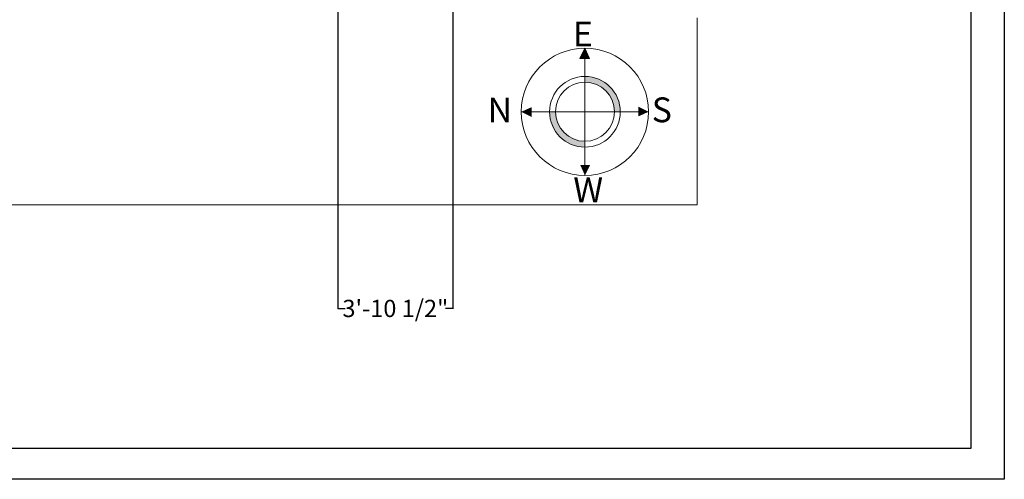
# Model space of a CAD drawing. Units: inches. Extents: x 0 to 4258, y 0 to 3769.
# Tile 17 of 30: x 3859 to 4258, y 2750 to 2936. Entities that reach past the tile are written whole.
import ezdxf

# ---------------------------------------------------------------- set-up
doc = ezdxf.new("R2010")
doc.units = ezdxf.units.IN
doc.header["$MEASUREMENT"] = 0
for name, color, linetype, lineweight in [('A-ANNO-DIMS', 250, 'Continuous', 18), ('A-ANNO-SYMB', 250, 'Continuous', 18), ('A-ANNO-TTLB', 250, 'Continuous', 25), ('C-ROAD', 250, 'Continuous', 18)]:
    doc.layers.add(name, color=color, linetype=linetype, lineweight=lineweight)
doc.styles.get("Standard").update_dxf_attribs({"font": 'arial.ttf'})
doc.dimstyles.get("Standard").update_dxf_attribs({"dimtxt": 7, "dimasz": 0.18, "dimexe": 0.18, "dimexo": 0.0625, "dimgap": 0.09, "dimtad": 0, "dimtih": 1, "dimtoh": 1, "dimzin": 0, "dimdsep": 46, "dimlunit": 3, "dimtxsty": 'Standard', "dimcen": 0.09, "dimadec": 0, "dimazin": 0, "dimtfac": 1, "dimtofl": 0, "dimtmove": 0, "dimatfit": 3, "dimfxl": 1, "dimtolj": 1, "dimtzin": 0, "dimarcsym": 0})

# ---------------------------------------------------------------- blocks, each defined once
blk = doc.blocks.new('*D72')
at = {"layer": 'A-ANNO-DIMS', "color": 0, "lineweight": -2, "transparency": 16777216}
for p, q in [((4034.3, 3256.23), (4034.3, 2818.78)), ((3987.71, 3253.71), (3987.71, 2818.78)), ((3987.89, 2818.96), (3990.74, 2818.96)), ((4034.12, 2818.96), (4031.27, 2818.96))]:
    blk.add_line(p, q, dxfattribs=at)
at = {"layer": 'A-ANNO-DIMS', "color": 0, "transparency": 16777216}
for points in [[(3987.89, 2818.99), (3987.89, 2818.93), (3987.71, 2818.96)], [(4034.12, 2818.99), (4034.12, 2818.93), (4034.3, 2818.96)]]:
    blk.add_solid(points, dxfattribs=at)
at = {"layer": 'Defpoints', "color": 0, "transparency": 16777216}
for p in [(4034.3, 3256.29), (3987.71, 3253.78), (4034.3, 2818.96)]:
    blk.add_point(p, dxfattribs=at)
at = {"layer": 'A-ANNO-DIMS', "color": 0, "transparency": 16777216, "insert": (4011.01, 2818.96), "char_height": 7, "attachment_point": 5}
blk.add_mtext('\\A1;3\'-10 1/2"', dxfattribs=at)

msp = doc.modelspace()

# ---------------------------------------------------------------- hatches: boundary and pattern name
at = {"layer": 'A-ANNO-SYMB'}
h = msp.add_hatch(color=256, dxfattribs=at)
h.dxf.hatch_style = 1
h.paths.add_polyline_path([(4087.8, 2924.432), (4085.729, 2920.281), (4087.8, 2920.281)])
h.paths.add_polyline_path([(4087.8, 2924.432), (4087.8, 2920.281), (4089.664, 2920.281)])
h = msp.add_hatch(color=256, dxfattribs=at)
h.dxf.hatch_style = 1
h.paths.add_polyline_path([(4075.84, 2898.657), (4073.481, 2898.657, 0.4142136), (4087.8, 2884.338), (4087.8, 2886.698, -0.4142136)])
h.paths.add_polyline_path([(4087.8, 2912.976), (4087.8, 2910.616, -0.4142136), (4099.759, 2898.657), (4102.119, 2898.657, 0.4142136)])
h = msp.add_hatch(color=256, dxfattribs=at)
h.dxf.hatch_style = 1
h.paths.add_polyline_path([(4062.027, 2898.658), (4066.178, 2896.588), (4066.178, 2898.658)])
h.paths.add_polyline_path([(4062.027, 2898.658), (4066.178, 2898.658), (4066.178, 2900.523)])
h = msp.add_hatch(color=256, dxfattribs=at)
h.dxf.hatch_style = 1
h.paths.add_polyline_path([(4113.581, 2898.66), (4109.43, 2900.731), (4109.43, 2898.66)])
h.paths.add_polyline_path([(4113.581, 2898.66), (4109.43, 2898.66), (4109.43, 2896.795)])
h = msp.add_hatch(color=256, dxfattribs=at)
h.dxf.hatch_style = 1
h.paths.add_polyline_path([(4087.798, 2872.882), (4089.869, 2877.033), (4087.798, 2877.033)])
h.paths.add_polyline_path([(4087.798, 2872.882), (4087.798, 2877.033), (4085.934, 2877.033)])

# ---------------------------------------------------------------- linework, layer by layer
for p, q in [((4087.8, 2924.432), (4085.729, 2920.281)), ((4087.8, 2924.432), (4087.8, 2872.882)), ((4089.664, 2920.281), (4087.8, 2924.432)), ((4085.729, 2920.281), (4089.664, 2920.281)), ((4087.8, 2910.616), (4087.8, 2912.976)), ((4062.025, 2898.657), (4113.574, 2898.657)), ((4073.481, 2898.657), (4075.84, 2898.657)), ((4099.759, 2898.657), (4102.119, 2898.657)), ((4087.8, 2886.698), (4087.8, 2884.338))]:
    msp.add_line(p, q, dxfattribs=at)
for radius in [25.775, 14.319, 11.959]:
    msp.add_circle((4087.8, 2898.657), radius, dxfattribs=at)
at = {"layer": 'A-ANNO-TTLB'}
for p, q in [((4257.673, 3768.679), (4257.673, 2749.714)), ((4244.279, 2762.335), (4244.279, 3758.41)), ((3489.722, 2762.335), (4244.279, 2762.335)), ((4257.673, 2749.714), (3476.156, 2749.714))]:
    msp.add_line(p, q, dxfattribs=at)
at = {"layer": 'C-ROAD'}
for p, q in [((4133.199, 2860.957), (4133.199, 2936.793)), ((3596.728, 2860.957), (4133.199, 2860.957))]:
    msp.add_line(p, q, dxfattribs=at)

# ---------------------------------------------------------------- texts
at = {"layer": 'A-ANNO-SYMB'}
for s, p in [('E', (4082.925, 2925.119)), ('N', (4048.386, 2894.332)), ('S', (4114.856, 2894.428)), ('W', (4083.099, 2861.99))]:
    msp.add_text(s, height=10.057, dxfattribs=at).set_placement(p)

# ---------------------------------------------------------------- dimensions: what is measured, and where the dimension line sits
at = {"layer": 'A-ANNO-DIMS'}
dim = msp.add_linear_dim(base=(4034.304, 2818.957), p1=(3987.712, 3253.777), p2=(4034.304, 3256.293), dimstyle='Standard', override={"dimdec": 1, "dimlfac": 1, "dimrnd": 0, "dimzin": 1, "dimdsep": 46, "dimlunit": 4, "dimfrac": 2}, dxfattribs=at)
dim.commit()
dim.dimension.update_dxf_attribs({"geometry": '*D72', "text_midpoint": (4011.008, 2818.957)})

doc.saveas('drawing.dxf')
